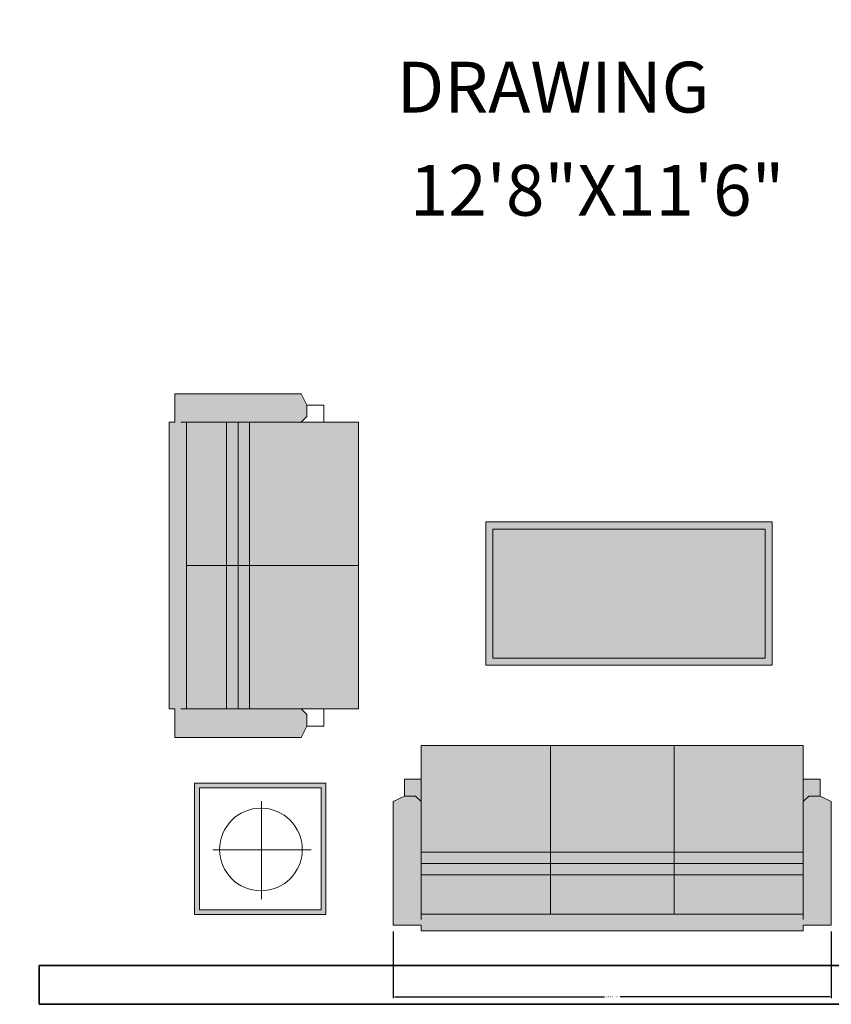
# Model space of a CAD drawing. Units: millimetres. Extents: x 27017497 to 27018854, y 7058029 to 7059154.
# Tile 52 of 91: x 27017886 to 27017980, y 7058294 to 7058409. Entities that reach past the tile are written whole.
import ezdxf

# ---------------------------------------------------------------- set-up
doc = ezdxf.new("R2010")
doc.units = ezdxf.units.MM
for name, color, linetype, lineweight in [('A-ANNO-DIMS', 2, 'Continuous', 18), ('A-AREA-IDEN', 7, 'Continuous', 18), ('A-FURN', 8, 'Continuous', 18), ('A-WALL', 7, 'Continuous', 35)]:
    doc.layers.add(name, color=color, linetype=linetype, lineweight=lineweight)
doc.layers.add('A-FURN-PATT', color=177, linetype='Continuous', lineweight=13, true_color=0x293189)
doc.styles.get("Standard").update_dxf_attribs({"font": 'arial.ttf'})
doc.dimstyles.get("Standard").update_dxf_attribs({"dimtxt": 0.18, "dimasz": 0.18, "dimexe": 0.18, "dimexo": 0.0625, "dimgap": 0.09, "dimtad": 0, "dimtih": 1, "dimtoh": 1, "dimdec": 4, "dimzin": 0, "dimdsep": 46, "dimtxsty": 'Standard', "dimcen": 0.09, "dimadec": 0, "dimazin": 0, "dimtfac": 1, "dimtdec": 4, "dimtofl": 0, "dimtmove": 0, "dimatfit": 3, "dimfxl": 1, "dimtolj": 1, "dimtzin": 0, "dimarcsym": 0})

# ---------------------------------------------------------------- blocks, each defined once
blk = doc.blocks.new('SOFA-THREE-SEAT')
for p, q in [((47.73, 21.58), (3.27, 21.58)), ((3.27, 21.58), (3.27, 17.65)), ((18.31, 21.58), (18.31, 1.96)), ((32.69, 21.58), (32.69, 1.96)), ((47.73, 17.65), (47.73, 21.58)), ((3.27, 17.65), (1.31, 17.65)), ((1.31, 17.65), (1.31, 15.69)), ((3.27, 17.65), (3.27, 15.04)), ((47.73, 17.65), (47.73, 15.04)), ((49.69, 17.65), (47.73, 17.65)), ((49.69, 15.69), (49.69, 17.65)), ((1.31, 15.69), (0, 15.04)), ((0, 15.04), (0, 0.65)), ((1.31, 15.69), (2.62, 15.69)), ((2.62, 15.69), (3.27, 15.04)), ((3.27, 15.04), (3.27, 1.31)), ((48.38, 15.69), (47.73, 15.04)), ((47.73, 15.04), (47.73, 1.31)), ((49.69, 15.69), (48.38, 15.69)), ((51, 15.04), (49.69, 15.69)), ((51, 0.65), (51, 15.04)), ((47.73, 9.15), (3.27, 9.15)), ((47.73, 7.85), (3.27, 7.85)), ((47.73, 6.54), (3.27, 6.54)), ((3.27, 1.96), (47.73, 1.96)), ((0, 0.65), (3.27, 0.65)), ((3.27, 0.65), (3.27, 0)), ((47.73, 0), (47.73, 0.65)), ((47.73, 0.65), (51, 0.65)), ((3.27, 0), (47.73, 0))]:
    blk.add_line(p, q)
blk = doc.blocks.new('SETTEE-TWO-SEAT')
for p, q in [((6.67, 40.01), (6, 38.68)), ((21.34, 40.01), (6.67, 40.01)), ((21.34, 36.68), (21.34, 40.01)), ((6, 38.68), (4, 38.68)), ((4, 38.68), (4, 36.68)), ((6, 38.68), (6, 37.35)), ((0, 36.68), (0, 3.33)), ((4, 36.68), (0, 36.68)), ((4, 36.68), (6.67, 36.68)), ((6, 37.35), (6.67, 36.68)), ((6.67, 36.68), (20.67, 36.68)), ((12.67, 36.68), (12.67, 3.33)), ((14, 36.68), (14, 3.33)), ((15.34, 36.68), (15.34, 3.33)), ((20.01, 3.33), (20.01, 36.68)), ((22.01, 36.68), (21.34, 36.68)), ((22.01, 3.33), (22.01, 36.68)), ((0, 20.01), (20.01, 20.01)), ((0, 3.33), (4, 3.33)), ((4, 3.33), (6.67, 3.33)), ((4, 3.33), (4, 1.33)), ((6, 2.67), (6.67, 3.33)), ((6, 1.33), (6, 2.67)), ((6.67, 3.33), (20.67, 3.33)), ((21.34, 0), (21.34, 3.33)), ((21.34, 3.33), (22.01, 3.33)), ((4, 1.33), (6, 1.33)), ((6, 1.33), (6.67, 0)), ((6.67, 0), (21.34, 0))]:
    blk.add_line(p, q)
blk = doc.blocks.new('TABLE-END')
for p, q in [((15.28, 15.28), (0, 15.28)), ((0, 15.28), (0, 0)), ((15.28, 0), (15.28, 15.28)), ((14.73, 14.73), (0.56, 14.73)), ((0.56, 14.73), (0.56, 0.56)), ((14.73, 0.56), (14.73, 14.73)), ((7.79, 1.78), (7.79, 13.18)), ((2.12, 7.51), (13.57, 7.51)), ((0.56, 0.56), (14.73, 0.56)), ((0, 0), (15.28, 0))]:
    blk.add_line(p, q)
blk.add_circle((7.72, 7.57), 4.81)
blk = doc.blocks.new('TABLE-COFFEE')
for p, q in [((33.35, 16.67), (0, 16.67)), ((0, 16.67), (0, 0)), ((33.35, 0), (33.35, 16.67)), ((32.51, 15.84), (0.83, 15.84)), ((0.83, 15.84), (0.83, 0.83)), ((32.51, 0.83), (32.51, 15.84)), ((0, 0), (33.35, 0)), ((0.83, 0.83), (32.51, 0.83))]:
    blk.add_line(p, q)
blk = doc.blocks.new('*D37')
at = {"layer": 'A-ANNO-DIMS', "color": 0, "lineweight": -2, "transparency": 16777216}
for p, q in [((27017929.38, 7058302.89), (27017929.38, 7058295.12)), ((27017980.38, 7058302.89), (27017980.38, 7058295.12)), ((27017929.56, 7058295.3), (27017953.98, 7058295.3)), ((27017980.2, 7058295.3), (27017955.79, 7058295.3))]:
    blk.add_line(p, q, dxfattribs=at)
at = {"layer": 'A-ANNO-DIMS', "color": 0, "transparency": 16777216}
for points in [[(27017929.56, 7058295.33), (27017929.56, 7058295.27), (27017929.38, 7058295.3)], [(27017980.2, 7058295.33), (27017980.2, 7058295.27), (27017980.38, 7058295.3)]]:
    blk.add_solid(points, dxfattribs=at)
at = {"layer": 'Defpoints', "color": 0, "transparency": 16777216}
for p in [(27017929.38, 7058302.95), (27017980.38, 7058302.95), (27017980.38, 7058295.3)]:
    blk.add_point(p, dxfattribs=at)
at = {"layer": 'A-ANNO-DIMS', "color": 0, "transparency": 16777216, "insert": (27017954.88, 7058295.3), "char_height": 0.18, "attachment_point": 5}
blk.add_mtext('\\A1;SOFA 51 TYP.', dxfattribs=at)
blk = doc.blocks.new('*D48')
at = {"layer": 'A-ANNO-DIMS', "color": 0, "lineweight": -2, "transparency": 16777216}
for p, q in [((27018463.5, 7058622.91), (27017497.54, 7058622.91)), ((27017497.72, 7058622.73), (27017497.72, 7058357.75)), ((27017497.72, 7058092.41), (27017497.72, 7058357.39)), ((27018555.13, 7058092.23), (27017497.54, 7058092.23))]:
    blk.add_line(p, q, dxfattribs=at)
at = {"layer": 'A-ANNO-DIMS', "color": 0, "transparency": 16777216}
for points in [[(27017497.69, 7058622.73), (27017497.75, 7058622.73), (27017497.72, 7058622.91)], [(27017497.69, 7058092.41), (27017497.75, 7058092.41), (27017497.72, 7058092.23)]]:
    blk.add_solid(points, dxfattribs=at)
at = {"layer": 'Defpoints', "color": 0, "transparency": 16777216}
for p in [(27018463.56, 7058622.91), (27017497.72, 7058092.23), (27018555.19, 7058092.23)]:
    blk.add_point(p, dxfattribs=at)
at = {"layer": 'A-ANNO-DIMS', "color": 0, "transparency": 16777216, "insert": (27017497.72, 7058357.57), "char_height": 0.18, "attachment_point": 5}
blk.add_mtext('\\A1;530.7', dxfattribs=at)

msp = doc.modelspace()

# ---------------------------------------------------------------- hatches: boundary and pattern name
at = {"layer": 'A-FURN-PATT'}
h = msp.add_hatch(color=256, dxfattribs=at)
h.dxf.hatch_style = 1
h.paths.add_polyline_path([(27017921.559, 7058320.14), (27017906.276, 7058320.14), (27017906.276, 7058304.857), (27017921.559, 7058304.857)])
h.paths.add_polyline_path([(27017921.003, 7058319.584), (27017921.003, 7058305.412), (27017906.831, 7058305.412), (27017906.831, 7058319.584)], flags=16)
h.paths.add_polyline_path([(27017918.811, 7058312.427, -1), (27017909.19, 7058312.427, -1)], flags=0)
h.paths.add_polyline_path([(27017919.33, 7058326.783), (27017919.33, 7058328.117), (27017918.663, 7058328.784), (27017905.325, 7058328.784), (27017905.325, 7058362.129), (27017918.663, 7058362.129), (27017919.33, 7058362.796), (27017919.33, 7058364.13), (27017918.663, 7058365.463), (27017903.991, 7058365.463), (27017903.991, 7058362.129), (27017903.325, 7058362.129), (27017903.325, 7058328.784), (27017903.991, 7058328.784), (27017903.991, 7058325.45), (27017918.663, 7058325.45)])
h.paths.add_polyline_path([(27017925.332, 7058345.456), (27017912.661, 7058345.456), (27017912.661, 7058328.784), (27017918.663, 7058328.784), (27017921.331, 7058328.784), (27017925.332, 7058328.784)])
h.paths.add_polyline_path([(27017925.332, 7058362.129), (27017921.331, 7058362.129), (27017918.663, 7058362.129), (27017912.661, 7058362.129), (27017912.661, 7058345.456), (27017925.332, 7058345.456)])
h.paths.add_polyline_path([(27017909.993, 7058362.129), (27017905.325, 7058362.129), (27017905.325, 7058345.456), (27017909.993, 7058345.456)], flags=17)
h.paths.add_polyline_path([(27017909.993, 7058345.456), (27017905.325, 7058345.456), (27017905.325, 7058328.784), (27017909.993, 7058328.784)], flags=17)
h.paths.add_polyline_path([(27017911.327, 7058345.456), (27017909.993, 7058345.456), (27017909.993, 7058328.784), (27017911.327, 7058328.784)], flags=17)
h.paths.add_polyline_path([(27017912.661, 7058345.456), (27017911.327, 7058345.456), (27017911.327, 7058328.784), (27017912.661, 7058328.784)], flags=17)
h.paths.add_polyline_path([(27017912.661, 7058362.129), (27017911.327, 7058362.129), (27017911.327, 7058345.456), (27017912.661, 7058345.456)], flags=17)
h.paths.add_polyline_path([(27017911.327, 7058362.129), (27017909.993, 7058362.129), (27017909.993, 7058345.456), (27017911.327, 7058345.456)], flags=17)
h.paths.add_polyline_path([(27017973.504, 7058350.536), (27017940.159, 7058350.536), (27017940.159, 7058333.863), (27017973.504, 7058333.863)])
h.paths.add_polyline_path([(27017972.67, 7058349.702), (27017972.67, 7058334.697), (27017940.993, 7058334.697), (27017940.993, 7058349.702)], flags=16)
h.paths.add_polyline_path([(27018000.44, 7058364.252), (27017994.438, 7058364.252), (27017991.77, 7058364.252), (27017987.769, 7058364.252), (27017987.769, 7058347.58), (27018000.44, 7058347.58)])
h.paths.add_polyline_path([(27018000.44, 7058347.58), (27017987.769, 7058347.58), (27017987.769, 7058330.907), (27017991.77, 7058330.907), (27017994.438, 7058330.907), (27018000.44, 7058330.907)])
h.paths.add_polyline_path([(27018009.109, 7058330.907), (27018009.776, 7058330.907), (27018009.776, 7058364.252), (27018009.109, 7058364.252), (27018009.109, 7058367.587), (27017994.438, 7058367.587), (27017993.771, 7058366.253), (27017993.771, 7058364.919), (27017994.438, 7058364.252), (27018007.775, 7058364.252), (27018007.775, 7058330.907), (27017994.438, 7058330.907), (27017993.771, 7058330.241), (27017993.771, 7058328.907), (27017994.438, 7058327.573), (27018009.109, 7058327.573)])
h.paths.add_polyline_path([(27017994.438, 7058330.907), (27017991.77, 7058330.907), (27017991.77, 7058328.907), (27017993.771, 7058328.907), (27017993.771, 7058330.241)])
h.paths.add_polyline_path([(27017993.771, 7058366.253), (27017991.77, 7058366.253), (27017991.77, 7058364.252), (27017994.438, 7058364.252), (27017993.771, 7058364.919)])
h.paths.add_polyline_path([(27018007.775, 7058364.252), (27018003.107, 7058364.252), (27018003.107, 7058347.58), (27018007.775, 7058347.58)], flags=17)
h.paths.add_polyline_path([(27018007.775, 7058347.58), (27018003.107, 7058347.58), (27018003.107, 7058330.907), (27018007.775, 7058330.907)], flags=17)
h.paths.add_polyline_path([(27018003.107, 7058364.252), (27018001.773, 7058364.252), (27018001.773, 7058347.58), (27018003.107, 7058347.58)], flags=17)
h.paths.add_polyline_path([(27018003.107, 7058347.58), (27018001.773, 7058347.58), (27018001.773, 7058330.907), (27018003.107, 7058330.907)], flags=17)
h.paths.add_polyline_path([(27018001.773, 7058347.58), (27018000.44, 7058347.58), (27018000.44, 7058330.907), (27018001.773, 7058330.907)], flags=17)
h.paths.add_polyline_path([(27018001.773, 7058364.252), (27018000.44, 7058364.252), (27018000.44, 7058347.58), (27018001.773, 7058347.58)], flags=17)
h = msp.add_hatch(color=256, dxfattribs=at)
h.dxf.hatch_style = 1
h.paths.add_polyline_path([(27017972.67, 7058349.702), (27017940.993, 7058349.702), (27017940.993, 7058334.697), (27017972.67, 7058334.697)])
h.paths.add_polyline_path([(27017962.073, 7058324.531), (27017947.689, 7058324.531), (27017947.689, 7058312.108), (27017962.073, 7058312.108)])
h.paths.add_polyline_path([(27017977.111, 7058320.608), (27017977.111, 7058324.531), (27017962.073, 7058324.531), (27017962.073, 7058312.108), (27017977.111, 7058312.108), (27017977.111, 7058317.992)])
h.paths.add_polyline_path([(27017947.689, 7058324.531), (27017932.651, 7058324.531), (27017932.651, 7058320.608), (27017932.651, 7058317.992), (27017932.651, 7058312.108), (27017947.689, 7058312.108)])
h.paths.add_polyline_path([(27017932.651, 7058317.992), (27017931.997, 7058318.646), (27017930.69, 7058318.646), (27017929.382, 7058317.992), (27017929.382, 7058303.608), (27017932.651, 7058303.608), (27017932.651, 7058302.955), (27017977.111, 7058302.955), (27017977.111, 7058303.608), (27017980.38, 7058303.608), (27017980.38, 7058317.992), (27017979.072, 7058318.646), (27017977.765, 7058318.646), (27017977.111, 7058317.992), (27017977.111, 7058304.916), (27017932.651, 7058304.916)])
h.paths.add_polyline_path([(27017947.689, 7058312.108), (27017932.651, 7058312.108), (27017932.651, 7058310.8), (27017947.689, 7058310.8)], flags=17)
h.paths.add_polyline_path([(27017962.073, 7058312.108), (27017947.689, 7058312.108), (27017947.689, 7058310.8), (27017962.073, 7058310.8)], flags=17)
h.paths.add_polyline_path([(27017977.111, 7058312.108), (27017962.073, 7058312.108), (27017962.073, 7058310.8), (27017977.111, 7058310.8)], flags=17)
h.paths.add_polyline_path([(27017977.111, 7058310.8), (27017962.073, 7058310.8), (27017962.073, 7058309.493), (27017977.111, 7058309.493)], flags=17)
h.paths.add_polyline_path([(27017962.073, 7058310.8), (27017947.689, 7058310.8), (27017947.689, 7058309.493), (27017962.073, 7058309.493)], flags=17)
h.paths.add_polyline_path([(27017947.689, 7058310.8), (27017932.651, 7058310.8), (27017932.651, 7058309.493), (27017947.689, 7058309.493)], flags=17)
h.paths.add_polyline_path([(27017947.689, 7058309.493), (27017932.651, 7058309.493), (27017932.651, 7058304.916), (27017947.689, 7058304.916)], flags=17)
h.paths.add_polyline_path([(27017962.073, 7058309.493), (27017947.689, 7058309.493), (27017947.689, 7058304.916), (27017962.073, 7058304.916)], flags=17)
h.paths.add_polyline_path([(27017977.111, 7058309.493), (27017962.073, 7058309.493), (27017962.073, 7058304.916), (27017977.111, 7058304.916)], flags=17)
h.paths.add_polyline_path([(27017979.072, 7058320.608), (27017977.111, 7058320.608), (27017977.111, 7058317.992), (27017977.765, 7058318.646), (27017979.072, 7058318.646)])
h.paths.add_polyline_path([(27017932.651, 7058320.608), (27017930.69, 7058320.608), (27017930.69, 7058318.646), (27017931.997, 7058318.646), (27017932.651, 7058317.992)])
h.paths.add_polyline_path([(27018002.231, 7058320.14), (27017986.948, 7058320.14), (27017986.948, 7058304.857), (27018002.231, 7058304.857)])
h.paths.add_polyline_path([(27018001.676, 7058319.584), (27018001.676, 7058305.412), (27017987.504, 7058305.412), (27017987.504, 7058319.584)], flags=16)
h.paths.add_polyline_path([(27017999.483, 7058312.427, -1), (27017989.862, 7058312.427, -1)], flags=0)

# ---------------------------------------------------------------- linework, layer by layer
at = {"layer": 'A-WALL'}
for p, q in [((27017888.166, 7058298.912), (27017888.166, 7058294.412)), ((27017888.166, 7058298.912), (27018032.166, 7058298.912)), ((27017888.166, 7058294.412), (27018032.166, 7058294.412))]:
    msp.add_line(p, q, dxfattribs=at)

# ---------------------------------------------------------------- block references
at = {"layer": 'A-FURN', "extrusion": (0, 0, -1), "zscale": -1}
msp.add_blockref('SETTEE-TWO-SEAT', (-27017925.332, 7058325.45), dxfattribs=at)
at = {"layer": 'A-FURN'}
for name, p in [('TABLE-COFFEE', (27017940.159, 7058333.863)), ('SOFA-THREE-SEAT', (27017929.382, 7058302.955)), ('TABLE-END', (27017906.276, 7058304.857))]:
    msp.add_blockref(name, p, dxfattribs=at)

# ---------------------------------------------------------------- texts
at = {"layer": 'A-ANNO-DIMS'}
msp.add_text('12\'8"X11\'6"', height=5.91176, dxfattribs=at).set_placement((27017931.317, 7058386.175))
at = {"layer": 'A-AREA-IDEN'}
msp.add_text('DRAWING', height=5.9118, dxfattribs=at).set_placement((27017929.782, 7058398.172))

# ---------------------------------------------------------------- dimensions: what is measured, and where the dimension line sits
at = {"layer": 'A-ANNO-DIMS'}
dim = msp.add_linear_dim(base=(27017497.716, 7058092.23), p1=(27018463.561, 7058622.912), p2=(27018555.192, 7058092.23), angle=90, dimstyle='Standard', override={"dimdec": 1, "dimlfac": 1, "dimrnd": 0, "dimzin": 0, "dimdsep": 46, "dimlunit": 2}, dxfattribs=at)
dim.commit()
dim.dimension.update_dxf_attribs({"geometry": '*D48', "text_midpoint": (27017497.716, 7058357.571)})
dim = msp.add_linear_dim(base=(27017980.38, 7058295.305), p1=(27017929.382, 7058302.955), p2=(27017980.38, 7058302.955), text='SOFA <> TYP.', dimstyle='Standard', override={"dimdec": 0, "dimlfac": 1, "dimrnd": 0, "dimzin": 0, "dimdsep": 46, "dimlunit": 2}, dxfattribs=at)
dim.commit()
dim.dimension.update_dxf_attribs({"geometry": '*D37', "text_midpoint": (27017954.881, 7058295.305)})

doc.saveas('drawing.dxf')
